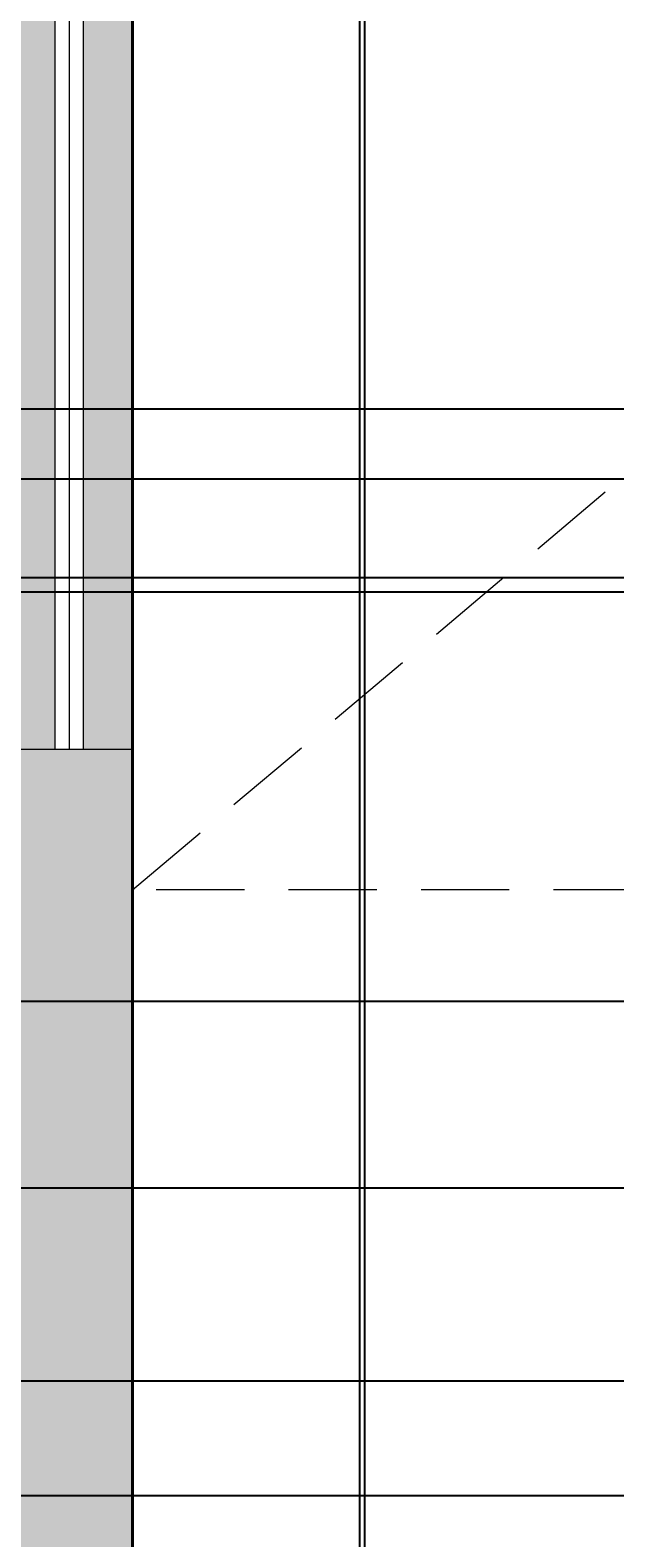
# Model space of a CAD drawing. Units: inches. Extents: x 818 to 1898, y 976 to 2364.
# Tile 67 of 96: x 1260 to 1302, y 1873 to 1980. Entities that reach past the tile are written whole.
import ezdxf

# ---------------------------------------------------------------- set-up
doc = ezdxf.new("R2010")
doc.units = ezdxf.units.IN
doc.header["$LTSCALE"] = 5
doc.header["$MEASUREMENT"] = 0
doc.linetypes.add('HIDDEN', pattern=[0.375, 0.25, -0.125])
for name, color, linetype, lineweight in [('A-ANNO-DIMS', 2, 'Continuous', 18), ('A-FLOR-OVHD', 8, 'HIDDEN', 13), ('A-GLAZ', 4, 'Continuous', 18), ('A-WALL', 7, 'Continuous', 40)]:
    doc.layers.add(name, color=color, linetype=linetype, lineweight=lineweight)
doc.layers.add('A-GLAZ-PATT', color=141, linetype='Continuous', lineweight=9, true_color=0xadddf7)
doc.layers.add('A-WALL-PATT', color=251, linetype='Continuous', lineweight=13, true_color=0x636466)
doc.styles.get("Standard").update_dxf_attribs({"font": 'arial.ttf'})
doc.dimstyles.get("Standard").update_dxf_attribs({"dimtxt": 0.18, "dimasz": 0.18, "dimexe": 0.18, "dimexo": 0.0625, "dimgap": 0.09, "dimtad": 0, "dimtih": 1, "dimtoh": 1, "dimdec": 4, "dimzin": 0, "dimdsep": 46, "dimtxsty": 'Standard', "dimcen": 0.09, "dimadec": 0, "dimazin": 0, "dimtfac": 1, "dimtdec": 4, "dimtofl": 0, "dimtmove": 0, "dimatfit": 3, "dimfxl": 1, "dimtolj": 1, "dimtzin": 0, "dimarcsym": 0})

# ---------------------------------------------------------------- blocks, each defined once
blk = doc.blocks.new('*D61')
at = {"layer": 'A-ANNO-DIMS', "color": 0, "lineweight": -2, "ltscale": 5, "transparency": 16777216}
for p, q in [((1071.73, 1203.03), (1071.73, 2363.87)), ((1071.91, 2363.69), (1250.94, 2363.69)), ((1430.55, 2363.69), (1251.51, 2363.69)), ((1430.73, 1203.03), (1430.73, 2363.87))]:
    blk.add_line(p, q, dxfattribs=at)
at = {"layer": 'A-ANNO-DIMS', "color": 0, "ltscale": 5, "transparency": 16777216}
for points in [[(1071.91, 2363.72), (1071.91, 2363.66), (1071.73, 2363.69)], [(1430.55, 2363.72), (1430.55, 2363.66), (1430.73, 2363.69)]]:
    blk.add_solid(points, dxfattribs=at)
at = {"layer": 'Defpoints', "color": 0, "ltscale": 5, "transparency": 16777216}
for p in [(1430.73, 2363.69), (1071.73, 1202.96), (1430.73, 1202.96)]:
    blk.add_point(p, dxfattribs=at)
at = {"layer": 'A-ANNO-DIMS', "color": 0, "ltscale": 5, "transparency": 16777216, "insert": (1251.23, 2363.69), "char_height": 0.18, "attachment_point": 5}
blk.add_mtext('\\A1;359', dxfattribs=at)
blk = doc.blocks.new('*D64')
at = {"layer": 'A-ANNO-DIMS', "color": 0, "lineweight": -2, "ltscale": 5, "transparency": 16777216}
for p, q in [((1197.73, 1501.14), (1197.73, 2363.87)), ((1197.91, 2363.69), (1313.93, 2363.69)), ((1430.55, 2363.69), (1314.52, 2363.69)), ((1430.73, 1501.14), (1430.73, 2363.87))]:
    blk.add_line(p, q, dxfattribs=at)
at = {"layer": 'A-ANNO-DIMS', "color": 0, "ltscale": 5, "transparency": 16777216}
for points in [[(1197.91, 2363.72), (1197.91, 2363.66), (1197.73, 2363.69)], [(1430.55, 2363.72), (1430.55, 2363.66), (1430.73, 2363.69)]]:
    blk.add_solid(points, dxfattribs=at)
at = {"layer": 'Defpoints', "color": 0, "ltscale": 5, "transparency": 16777216}
for p in [(1430.73, 2363.69), (1197.73, 1501.08), (1430.73, 1501.08)]:
    blk.add_point(p, dxfattribs=at)
at = {"layer": 'A-ANNO-DIMS', "color": 0, "ltscale": 5, "transparency": 16777216, "insert": (1314.23, 2363.69), "char_height": 0.18, "attachment_point": 5}
blk.add_mtext('\\A1;233', dxfattribs=at)
blk = doc.blocks.new('*D74')
at = {"layer": 'A-ANNO-DIMS', "color": 0, "lineweight": -2, "ltscale": 5, "transparency": 16777216}
for p, q in [((1590.66, 1940.08), (818.03, 1940.08)), ((818.21, 1939.9), (818.21, 1925.76)), ((818.21, 1911.26), (818.21, 1925.4)), ((1590.66, 1911.08), (818.03, 1911.08))]:
    blk.add_line(p, q, dxfattribs=at)
at = {"layer": 'A-ANNO-DIMS', "color": 0, "ltscale": 5, "transparency": 16777216}
for points in [[(818.18, 1939.9), (818.24, 1939.9), (818.21, 1940.08)], [(818.18, 1911.26), (818.24, 1911.26), (818.21, 1911.08)]]:
    blk.add_solid(points, dxfattribs=at)
at = {"layer": 'Defpoints', "color": 0, "ltscale": 5, "transparency": 16777216}
for p in [(818.21, 1940.08), (1590.73, 1940.08), (1590.73, 1911.08)]:
    blk.add_point(p, dxfattribs=at)
at = {"layer": 'A-ANNO-DIMS', "color": 0, "ltscale": 5, "transparency": 16777216, "insert": (818.21, 1925.58), "char_height": 0.18, "attachment_point": 5}
blk.add_mtext('\\A1;29', dxfattribs=at)
blk = doc.blocks.new('*D85')
at = {"layer": 'A-ANNO-DIMS', "color": 0, "lineweight": -2, "ltscale": 5, "transparency": 16777216}
for p, q in [((1258.79, 2053.08), (1897.92, 2053.08)), ((1897.74, 2052.9), (1897.74, 1876.76)), ((1897.74, 1700.26), (1897.74, 1876.4)), ((1258.79, 1700.08), (1897.92, 1700.08))]:
    blk.add_line(p, q, dxfattribs=at)
at = {"layer": 'A-ANNO-DIMS', "color": 0, "ltscale": 5, "transparency": 16777216}
for points in [[(1897.71, 2052.9), (1897.77, 2052.9), (1897.74, 2053.08)], [(1897.71, 1700.26), (1897.77, 1700.26), (1897.74, 1700.08)]]:
    blk.add_solid(points, dxfattribs=at)
at = {"layer": 'Defpoints', "color": 0, "ltscale": 5, "transparency": 16777216}
for p in [(1258.73, 2053.08), (1897.74, 2053.08), (1258.73, 1700.08)]:
    blk.add_point(p, dxfattribs=at)
at = {"layer": 'A-ANNO-DIMS', "color": 0, "ltscale": 5, "transparency": 16777216, "insert": (1897.74, 1876.58), "char_height": 0.18, "attachment_point": 5}
blk.add_mtext('\\A1;353', dxfattribs=at)
blk = doc.blocks.new('*D96')
at = {"layer": 'A-ANNO-DIMS', "color": 0, "lineweight": -2, "ltscale": 5, "transparency": 16777216}
for p, q in [((1229.65, 1071.12), (1229.65, 2363.87)), ((1229.83, 2363.69), (1256.52, 2363.69)), ((1283.99, 2363.69), (1257.3, 2363.69)), ((1284.17, 1071.12), (1284.17, 2363.87))]:
    blk.add_line(p, q, dxfattribs=at)
at = {"layer": 'A-ANNO-DIMS', "color": 0, "ltscale": 5, "transparency": 16777216}
for points in [[(1229.83, 2363.72), (1229.83, 2363.66), (1229.65, 2363.69)], [(1283.99, 2363.72), (1283.99, 2363.66), (1284.17, 2363.69)]]:
    blk.add_solid(points, dxfattribs=at)
at = {"layer": 'Defpoints', "color": 0, "ltscale": 5, "transparency": 16777216}
for p in [(1284.17, 2363.69), (1229.65, 1071.06), (1284.17, 1071.06)]:
    blk.add_point(p, dxfattribs=at)
at = {"layer": 'A-ANNO-DIMS', "color": 0, "ltscale": 5, "transparency": 16777216, "insert": (1256.91, 2363.69), "char_height": 0.18, "attachment_point": 5}
blk.add_mtext('\\A1;54.52', dxfattribs=at)
blk = doc.blocks.new('*D97')
at = {"layer": 'A-ANNO-DIMS', "color": 0, "lineweight": -2, "ltscale": 5, "transparency": 16777216}
for p, q in [((1284.17, 1071.12), (1284.17, 2363.87)), ((1284.35, 2363.69), (1310.96, 2363.69)), ((1338.36, 2363.69), (1311.75, 2363.69)), ((1338.54, 1071.12), (1338.54, 2363.87))]:
    blk.add_line(p, q, dxfattribs=at)
at = {"layer": 'A-ANNO-DIMS', "color": 0, "ltscale": 5, "transparency": 16777216}
for points in [[(1284.35, 2363.72), (1284.35, 2363.66), (1284.17, 2363.69)], [(1338.36, 2363.72), (1338.36, 2363.66), (1338.54, 2363.69)]]:
    blk.add_solid(points, dxfattribs=at)
at = {"layer": 'Defpoints', "color": 0, "ltscale": 5, "transparency": 16777216}
for p in [(1338.54, 2363.69), (1284.17, 1071.06), (1338.54, 1071.06)]:
    blk.add_point(p, dxfattribs=at)
at = {"layer": 'A-ANNO-DIMS', "color": 0, "ltscale": 5, "transparency": 16777216, "insert": (1311.36, 2363.69), "char_height": 0.18, "attachment_point": 5}
blk.add_mtext('\\A1;54.37', dxfattribs=at)
blk = doc.blocks.new('*D121')
at = {"layer": 'A-ANNO-DIMS', "color": 0, "lineweight": -2, "ltscale": 5, "transparency": 16777216}
for p, q in [((1766.29, 1884.2), (818.03, 1884.2)), ((818.21, 1884.02), (818.21, 1841.14)), ((818.21, 1797.9), (818.21, 1840.78)), ((1766.29, 1797.72), (818.03, 1797.72))]:
    blk.add_line(p, q, dxfattribs=at)
at = {"layer": 'A-ANNO-DIMS', "color": 0, "ltscale": 5, "transparency": 16777216}
for points in [[(818.18, 1884.02), (818.24, 1884.02), (818.21, 1884.2)], [(818.18, 1797.9), (818.24, 1797.9), (818.21, 1797.72)]]:
    blk.add_solid(points, dxfattribs=at)
at = {"layer": 'Defpoints', "color": 0, "ltscale": 5, "transparency": 16777216}
for p in [(818.21, 1884.2), (1766.35, 1884.2), (1766.35, 1797.72)]:
    blk.add_point(p, dxfattribs=at)
at = {"layer": 'A-ANNO-DIMS', "color": 0, "ltscale": 5, "transparency": 16777216, "insert": (818.21, 1840.96), "char_height": 0.18, "attachment_point": 5}
blk.add_mtext('\\A1;86.49', dxfattribs=at)
blk = doc.blocks.new('*D162')
at = {"layer": 'A-ANNO-DIMS', "color": 0, "lineweight": -2, "ltscale": 5, "transparency": 16777216}
for p, q in [((1429.16, 1876.08), (818.03, 1876.08)), ((818.21, 1875.9), (818.21, 1871.76)), ((818.21, 1867.26), (818.21, 1871.4)), ((1429.16, 1867.08), (818.03, 1867.08))]:
    blk.add_line(p, q, dxfattribs=at)
at = {"layer": 'A-ANNO-DIMS', "color": 0, "ltscale": 5, "transparency": 16777216}
for points in [[(818.18, 1875.9), (818.24, 1875.9), (818.21, 1876.08)], [(818.18, 1867.26), (818.24, 1867.26), (818.21, 1867.08)]]:
    blk.add_solid(points, dxfattribs=at)
at = {"layer": 'Defpoints', "color": 0, "ltscale": 5, "transparency": 16777216}
for p in [(1429.23, 1876.08), (818.21, 1867.08), (1429.23, 1867.08)]:
    blk.add_point(p, dxfattribs=at)
at = {"layer": 'A-ANNO-DIMS', "color": 0, "ltscale": 5, "transparency": 16777216, "insert": (818.21, 1871.58), "char_height": 0.18, "attachment_point": 5}
blk.add_mtext('\\A1;9', dxfattribs=at)
blk = doc.blocks.new('*D165')
at = {"layer": 'A-ANNO-DIMS', "color": 0, "lineweight": -2, "ltscale": 5, "transparency": 16777216}
for p, q in [((1283.82, 1510.14), (1283.82, 2363.87)), ((1284, 2363.69), (1324.09, 2363.69)), ((1364.97, 2363.69), (1324.88, 2363.69)), ((1365.15, 1510.14), (1365.15, 2363.87))]:
    blk.add_line(p, q, dxfattribs=at)
at = {"layer": 'A-ANNO-DIMS', "color": 0, "ltscale": 5, "transparency": 16777216}
for points in [[(1284, 2363.72), (1284, 2363.66), (1283.82, 2363.69)], [(1364.97, 2363.72), (1364.97, 2363.66), (1365.15, 2363.69)]]:
    blk.add_solid(points, dxfattribs=at)
at = {"layer": 'Defpoints', "color": 0, "ltscale": 5, "transparency": 16777216}
for p in [(1365.15, 2363.69), (1283.82, 1510.08), (1365.15, 1510.08)]:
    blk.add_point(p, dxfattribs=at)
at = {"layer": 'A-ANNO-DIMS', "color": 0, "ltscale": 5, "transparency": 16777216, "insert": (1324.48, 2363.69), "char_height": 0.18, "attachment_point": 5}
blk.add_mtext('\\A1;81.33', dxfattribs=at)
blk = doc.blocks.new('*D206')
at = {"layer": 'A-ANNO-DIMS', "color": 0, "lineweight": -2, "ltscale": 5, "transparency": 16777216}
for p, q in [((1590.66, 1911.08), (818.03, 1911.08)), ((818.21, 1910.9), (818.21, 1893.76)), ((818.21, 1876.26), (818.21, 1893.4)), ((1590.66, 1876.08), (818.03, 1876.08))]:
    blk.add_line(p, q, dxfattribs=at)
at = {"layer": 'A-ANNO-DIMS', "color": 0, "ltscale": 5, "transparency": 16777216}
for points in [[(818.18, 1910.9), (818.24, 1910.9), (818.21, 1911.08)], [(818.18, 1876.26), (818.24, 1876.26), (818.21, 1876.08)]]:
    blk.add_solid(points, dxfattribs=at)
at = {"layer": 'Defpoints', "color": 0, "ltscale": 5, "transparency": 16777216}
for p in [(818.21, 1911.08), (1590.73, 1911.08), (1590.73, 1876.08)]:
    blk.add_point(p, dxfattribs=at)
at = {"layer": 'A-ANNO-DIMS', "color": 0, "ltscale": 5, "transparency": 16777216, "insert": (818.21, 1893.58), "char_height": 0.18, "attachment_point": 5}
blk.add_mtext('\\A1;35', dxfattribs=at)
blk = doc.blocks.new('*D211')
at = {"layer": 'A-ANNO-DIMS', "color": 0, "lineweight": -2, "ltscale": 5, "transparency": 16777216}
for p, q in [((1599.66265, 1948.078237), (818.025912, 1948.078237)), ((818.205912, 1947.898237), (818.205912, 1944.758237)), ((818.205912, 1941.258237), (818.205912, 1944.398237)), ((1599.66265, 1941.078237), (818.025912, 1941.078237))]:
    blk.add_line(p, q, dxfattribs=at)
at = {"layer": 'A-ANNO-DIMS', "color": 0, "ltscale": 5, "transparency": 16777216}
for points in [[(818.175912, 1947.898237), (818.235912, 1947.898237), (818.205912, 1948.078237)], [(818.175912, 1941.258237), (818.235912, 1941.258237), (818.205912, 1941.078237)]]:
    blk.add_solid(points, dxfattribs=at)
at = {"layer": 'Defpoints', "color": 0, "ltscale": 5, "transparency": 16777216}
for p in [(818.205912, 1948.078237), (1599.72515, 1948.078237), (1599.72515, 1941.078237)]:
    blk.add_point(p, dxfattribs=at)
at = {"layer": 'A-ANNO-DIMS', "color": 0, "ltscale": 5, "transparency": 16777216, "insert": (818.205912, 1944.578237), "char_height": 0.18, "attachment_point": 5}
blk.add_mtext('\\A1;7', dxfattribs=at)
blk = doc.blocks.new('*D215')
at = {"layer": 'A-ANNO-DIMS', "color": 0, "lineweight": -2, "ltscale": 5, "transparency": 16777216}
for p, q in [((1590.66, 1876.08), (818.03, 1876.08)), ((818.21, 1875.9), (818.21, 1781.76)), ((818.21, 1687.26), (818.21, 1781.4)), ((1511.66, 1687.08), (818.03, 1687.08))]:
    blk.add_line(p, q, dxfattribs=at)
at = {"layer": 'A-ANNO-DIMS', "color": 0, "ltscale": 5, "transparency": 16777216}
for points in [[(818.18, 1875.9), (818.24, 1875.9), (818.21, 1876.08)], [(818.18, 1687.26), (818.24, 1687.26), (818.21, 1687.08)]]:
    blk.add_solid(points, dxfattribs=at)
at = {"layer": 'Defpoints', "color": 0, "ltscale": 5, "transparency": 16777216}
for p in [(818.21, 1876.08), (1590.73, 1876.08), (1511.73, 1687.08)]:
    blk.add_point(p, dxfattribs=at)
at = {"layer": 'A-ANNO-DIMS', "color": 0, "ltscale": 5, "transparency": 16777216, "insert": (818.21, 1781.58), "char_height": 0.18, "attachment_point": 5}
blk.add_mtext('\\A1;189', dxfattribs=at)
blk = doc.blocks.new('*D232')
at = {"layer": 'A-ANNO-DIMS', "color": 0, "lineweight": -2, "ltscale": 5, "transparency": 16777216}
for p, q in [((1303.87, 2008.39), (818.03, 2008.39)), ((818.21, 2008.21), (818.21, 1980.9)), ((818.21, 1953.22), (818.21, 1980.53)), ((1303.87, 1953.04), (818.03, 1953.04))]:
    blk.add_line(p, q, dxfattribs=at)
at = {"layer": 'A-ANNO-DIMS', "color": 0, "ltscale": 5, "transparency": 16777216}
for points in [[(818.18, 2008.21), (818.24, 2008.21), (818.21, 2008.39)], [(818.18, 1953.22), (818.24, 1953.22), (818.21, 1953.04)]]:
    blk.add_solid(points, dxfattribs=at)
at = {"layer": 'Defpoints', "color": 0, "ltscale": 5, "transparency": 16777216}
for p in [(818.21, 2008.39), (1303.93, 2008.39), (1303.93, 1953.04)]:
    blk.add_point(p, dxfattribs=at)
at = {"layer": 'A-ANNO-DIMS', "color": 0, "ltscale": 5, "transparency": 16777216, "insert": (818.21, 1980.72), "char_height": 0.18, "attachment_point": 5}
blk.add_mtext('\\A1;55.35', dxfattribs=at)
blk = doc.blocks.new('*D233')
at = {"layer": 'A-ANNO-DIMS', "color": 0, "lineweight": -2, "ltscale": 5, "transparency": 16777216}
for p, q in [((1267.73, 2044.02), (1267.73, 975.66)), ((1303.93, 2008.33), (1303.93, 975.66)), ((1267.91, 975.84), (1285.36, 975.84)), ((1303.75, 975.84), (1286.29, 975.84))]:
    blk.add_line(p, q, dxfattribs=at)
at = {"layer": 'A-ANNO-DIMS', "color": 0, "ltscale": 5, "transparency": 16777216}
for points in [[(1267.91, 975.87), (1267.91, 975.81), (1267.73, 975.84)], [(1303.75, 975.87), (1303.75, 975.81), (1303.93, 975.84)]]:
    blk.add_solid(points, dxfattribs=at)
at = {"layer": 'Defpoints', "color": 0, "ltscale": 5, "transparency": 16777216}
for p in [(1267.73, 2044.08), (1303.93, 2008.39), (1303.93, 975.84)]:
    blk.add_point(p, dxfattribs=at)
at = {"layer": 'A-ANNO-DIMS', "color": 0, "ltscale": 5, "transparency": 16777216, "insert": (1285.83, 975.84), "char_height": 0.18, "attachment_point": 5}
blk.add_mtext('\\A1;36.206', dxfattribs=at)
blk = doc.blocks.new('*D254')
at = {"layer": 'A-ANNO-DIMS', "color": 0, "lineweight": -2, "ltscale": 5, "transparency": 16777216}
for p, q in [((1267.73, 2044.02), (1267.73, 975.66)), ((1330.3, 2044.02), (1330.3, 975.66)), ((1267.91, 975.84), (1298.62, 975.84)), ((1330.12, 975.84), (1299.41, 975.84))]:
    blk.add_line(p, q, dxfattribs=at)
at = {"layer": 'A-ANNO-DIMS', "color": 0, "ltscale": 5, "transparency": 16777216}
for points in [[(1267.91, 975.87), (1267.91, 975.81), (1267.73, 975.84)], [(1330.12, 975.87), (1330.12, 975.81), (1330.3, 975.84)]]:
    blk.add_solid(points, dxfattribs=at)
at = {"layer": 'Defpoints', "color": 0, "ltscale": 5, "transparency": 16777216}
for p in [(1267.73, 2044.08), (1330.3, 2044.08), (1330.3, 975.84)]:
    blk.add_point(p, dxfattribs=at)
at = {"layer": 'A-ANNO-DIMS', "color": 0, "ltscale": 5, "transparency": 16777216, "insert": (1299.02, 975.84), "char_height": 0.18, "attachment_point": 5}
blk.add_mtext('\\A1;62.58', dxfattribs=at)
blk = doc.blocks.new('*D269')
at = {"layer": 'A-ANNO-DIMS', "color": 0, "lineweight": -2, "ltscale": 5, "transparency": 16777216}
for p, q in [((1246.94, 1534.14), (1246.94, 2363.87)), ((1247.12, 2363.69), (1293.71, 2363.69)), ((1341.08, 2363.69), (1294.49, 2363.69)), ((1341.26, 1534.14), (1341.26, 2363.87))]:
    blk.add_line(p, q, dxfattribs=at)
at = {"layer": 'A-ANNO-DIMS', "color": 0, "ltscale": 5, "transparency": 16777216}
for points in [[(1247.12, 2363.72), (1247.12, 2363.66), (1246.94, 2363.69)], [(1341.08, 2363.72), (1341.08, 2363.66), (1341.26, 2363.69)]]:
    blk.add_solid(points, dxfattribs=at)
at = {"layer": 'Defpoints', "color": 0, "ltscale": 5, "transparency": 16777216}
for p in [(1341.26, 2363.69), (1246.94, 1534.08), (1341.26, 1534.08)]:
    blk.add_point(p, dxfattribs=at)
at = {"layer": 'A-ANNO-DIMS', "color": 0, "ltscale": 5, "transparency": 16777216, "insert": (1294.1, 2363.69), "char_height": 0.18, "attachment_point": 5}
blk.add_mtext('\\A1;94.32', dxfattribs=at)
blk = doc.blocks.new('*D281')
at = {"layer": 'A-ANNO-DIMS', "color": 0, "lineweight": -2, "ltscale": 5, "transparency": 16777216}
for p, q in [((1250.3, 1913.7), (1250.3, 2363.87)), ((1250.48, 2363.69), (1420.12, 2363.69)), ((1590.55, 2363.69), (1420.91, 2363.69)), ((1590.73, 2011.14), (1590.73, 2363.87))]:
    blk.add_line(p, q, dxfattribs=at)
at = {"layer": 'A-ANNO-DIMS', "color": 0, "ltscale": 5, "transparency": 16777216}
for points in [[(1250.48, 2363.72), (1250.48, 2363.66), (1250.3, 2363.69)], [(1590.55, 2363.72), (1590.55, 2363.66), (1590.73, 2363.69)]]:
    blk.add_solid(points, dxfattribs=at)
at = {"layer": 'Defpoints', "color": 0, "ltscale": 5, "transparency": 16777216}
for p in [(1590.73, 2363.69), (1590.73, 2011.08), (1250.3, 1913.64)]:
    blk.add_point(p, dxfattribs=at)
at = {"layer": 'A-ANNO-DIMS', "color": 0, "ltscale": 5, "transparency": 16777216, "insert": (1420.51, 2363.69), "char_height": 0.18, "attachment_point": 5}
blk.add_mtext('\\A1;340.4', dxfattribs=at)
blk = doc.blocks.new('*D287')
at = {"layer": 'A-ANNO-DIMS', "color": 0, "lineweight": -2, "ltscale": 5, "transparency": 16777216}
for p, q in [((1303.87, 1953.04), (818.03, 1953.04)), ((818.21, 1952.86), (818.21, 1925.64)), ((818.21, 1898.05), (818.21, 1925.27)), ((1310.96, 1897.87), (818.03, 1897.87))]:
    blk.add_line(p, q, dxfattribs=at)
at = {"layer": 'A-ANNO-DIMS', "color": 0, "ltscale": 5, "transparency": 16777216}
for points in [[(818.18, 1952.86), (818.24, 1952.86), (818.21, 1953.04)], [(818.18, 1898.05), (818.24, 1898.05), (818.21, 1897.87)]]:
    blk.add_solid(points, dxfattribs=at)
at = {"layer": 'Defpoints', "color": 0, "ltscale": 5, "transparency": 16777216}
for p in [(818.21, 1953.04), (1303.93, 1953.04), (1311.03, 1897.87)]:
    blk.add_point(p, dxfattribs=at)
at = {"layer": 'A-ANNO-DIMS', "color": 0, "ltscale": 5, "transparency": 16777216, "insert": (818.21, 1925.45), "char_height": 0.18, "attachment_point": 5}
blk.add_mtext('\\A1;55.17', dxfattribs=at)

msp = doc.modelspace()

# ---------------------------------------------------------------- hatches: boundary and pattern name
at = {"layer": 'A-GLAZ-PATT', "ltscale": 5}
h = msp.add_hatch(color=256, dxfattribs=at)
h.dxf.hatch_style = 1
h.paths.add_polyline_path([(1283.8183, 1504.5782), (1206.7252, 1504.5782), (1206.7252, 1501.0782), (1283.8183, 1501.0782)])
h.paths.add_polyline_path([(1283.8183, 1510.0782), (1206.7252, 1510.0782), (1206.7252, 1506.5782), (1283.8183, 1506.5782)])
h.paths.add_polyline_path([(1490.9163, 1355.0782), (1439.7252, 1355.0782), (1439.7252, 1409.0522), (1436.2252, 1409.0522), (1436.2252, 1351.5782), (1490.9163, 1351.5782)])
h.paths.add_polyline_path([(1434.2252, 1409.0522), (1430.7251, 1409.0522), (1430.7251, 1346.0782), (1435.0799, 1346.0782), (1435.0731, 1346.1152), (1435.1501, 1346.0782), (1490.9163, 1346.0782), (1490.9163, 1349.5782), (1434.2252, 1349.5782)])
h.paths.add_polyline_path([(1714.7252, 1545.0782), (1711.2252, 1545.0782), (1711.2252, 1521.0782), (1714.7252, 1521.0782)])
h.paths.add_polyline_path([(1709.2252, 1545.0782), (1705.7252, 1545.0782), (1705.7252, 1521.0782), (1709.2252, 1521.0782)])
h.paths.add_polyline_path([(1714.7252, 1687.0782), (1711.2252, 1687.0782), (1711.2252, 1649.9029), (1714.7252, 1649.9029)])
h.paths.add_polyline_path([(1709.2252, 1687.0782), (1705.7252, 1687.0782), (1705.7252, 1649.9029), (1709.2252, 1649.9029)])
h.paths.add_polyline_path([(1709.2252, 1745.5584), (1705.7252, 1745.5584), (1705.7252, 1717.3178), (1709.2252, 1717.3178)])
h.paths.add_polyline_path([(1714.7252, 1745.5584), (1711.2252, 1745.5584), (1711.2252, 1717.3178), (1714.7252, 1717.3178)])
h.paths.add_polyline_path([(1714.7252, 2014.5114), (1711.2252, 2014.5114), (1711.2252, 1962.0338), (1714.7252, 1962.0338)])
h.paths.add_polyline_path([(1709.2252, 2014.5114), (1705.7252, 2014.5114), (1705.7252, 1962.0338), (1709.2252, 1962.0338)])
h.paths.add_polyline_path([(1538.5155, 2047.5782), (1485.1216, 2047.5782), (1485.1216, 2044.0782), (1538.5155, 2044.0782)])
h.paths.add_polyline_path([(1538.5155, 2053.0782), (1485.1216, 2053.0782), (1485.1216, 2049.5782), (1538.5155, 2049.5782)])
h.paths.add_polyline_path([(1388.0315, 2047.5782), (1330.305, 2047.5782), (1330.305, 2044.0782), (1388.0315, 2044.0782)])
h.paths.add_polyline_path([(1388.0315, 2053.0782), (1330.305, 2053.0782), (1330.305, 2049.5782), (1388.0315, 2049.5782)])
h.paths.add_polyline_path([(1262.2252, 2019.2871), (1258.7251, 2019.2871), (1258.7251, 1928.9218), (1262.2252, 1928.9218)])
h.paths.add_polyline_path([(1267.7251, 2019.2871), (1264.2252, 2019.2871), (1264.2252, 1928.9218), (1267.7251, 1928.9218)])
h.paths.add_polyline_path([(1262.2252, 1862.9652), (1258.7251, 1862.9652), (1258.7251, 1814.9652), (1262.2252, 1814.9652)])
h.paths.add_polyline_path([(1267.7251, 1862.9652), (1264.2252, 1862.9652), (1264.2252, 1814.9652), (1267.7251, 1814.9652)])
h.paths.add_polyline_path([(1262.2252, 1755.3321), (1258.7251, 1755.3321), (1258.7251, 1707.3321), (1262.2252, 1707.3321)])
h.paths.add_polyline_path([(1267.7251, 1755.3321), (1264.2252, 1755.3321), (1264.2252, 1707.3321), (1267.7251, 1707.3321)])
h.paths.add_polyline_path([(1251.9333, 1692.5782), (1206.7252, 1692.5782), (1206.7252, 1687.0782), (1251.9333, 1687.0782)])
h.paths.add_polyline_path([(1251.9333, 1700.0782), (1206.7252, 1700.0782), (1206.7252, 1694.5782), (1251.9333, 1694.5782)])
at = {"layer": 'A-WALL-PATT', "ltscale": 5}
h = msp.add_hatch(color=256, dxfattribs=at)
h.dxf.hatch_style = 1
h.paths.add_polyline_path([(1267.7251, 1928.9218), (1258.7251, 1928.9218), (1258.7251, 1913.6401), (1250.3029, 1913.6401), (1250.3029, 1878.3919), (1258.7251, 1878.3919), (1258.7251, 1862.9652), (1267.7251, 1862.9652)])
h.paths.add_polyline_path([(1267.7251, 1814.9652), (1258.7251, 1814.9652), (1258.7251, 1755.3321), (1267.7251, 1755.3321)])
h.paths.add_polyline_path([(1463.7252, 1696.0782), (1267.7251, 1696.0782), (1267.7251, 1707.3321), (1258.7251, 1707.3321), (1258.7251, 1700.0782), (1251.9333, 1700.0782), (1251.9333, 1687.0782), (1463.7252, 1687.0782)])
h.paths.add_polyline_path([(1714.7252, 1717.3178), (1705.7252, 1717.3178), (1705.7252, 1696.0782), (1599.7251, 1696.0782), (1599.7251, 1790.0782), (1705.7252, 1790.0782), (1705.7252, 1785.6125), (1714.7252, 1785.6125), (1714.7252, 1827.2125), (1705.7252, 1827.2125), (1705.7252, 1802.0782), (1599.7251, 1802.0782), (1599.7251, 1867.0782), (1705.7252, 1867.0782), (1705.7252, 1857.2125), (1714.7252, 1857.2125), (1714.7252, 1930.0316), (1741.8409, 1930.0316), (1741.8409, 1935.0316), (1714.7252, 1935.0316), (1714.7252, 1957.0338), (1741.8409, 1957.0338), (1741.8409, 1962.0338), (1714.7252, 1962.0338), (1705.7252, 1962.0338), (1705.7252, 1948.0782), (1599.7251, 1948.0782), (1599.7251, 1981.0782), (1590.7251, 1981.0782), (1590.7251, 1941.0782), (1620.7252, 1941.0782), (1705.7252, 1941.0782), (1705.7252, 1876.0782), (1599.7251, 1876.0782), (1599.7251, 1911.0782), (1590.7251, 1911.0782), (1590.7251, 1876.0782), (1429.2251, 1876.0782), (1429.2251, 1867.0782), (1511.7251, 1867.0782), (1528.593, 1867.0782), (1595.7252, 1867.0782), (1595.7252, 1773.0782), (1520.7252, 1773.0782), (1520.7252, 1837.5823), (1532.593, 1837.5823), (1532.593, 1867.0782), (1528.593, 1867.0782), (1528.593, 1841.5823), (1511.7251, 1841.5823), (1511.7251, 1744.9714), (1520.7252, 1744.9714), (1520.7252, 1761.0782), (1595.7252, 1761.0782), (1595.7252, 1696.0782), (1520.7252, 1696.0782), (1520.7252, 1716.0454), (1511.7251, 1716.0454), (1511.7251, 1696.0782), (1511.7251, 1687.0782), (1714.7252, 1687.0782)])
h.paths.add_polyline_path([(1714.7252, 2053.0782), (1714.7252, 2081.1881), (1709.7252, 2081.1881), (1709.7252, 2053.0782), (1681.6446, 2053.0782), (1681.6446, 2081.1881), (1676.6446, 2081.1881), (1676.6446, 2053.0782), (1538.5155, 2053.0782), (1538.5155, 2044.0782), (1590.7251, 2044.0782), (1590.7251, 2011.0782), (1599.7251, 2011.0782), (1599.7251, 2044.0782), (1705.7252, 2044.0782), (1705.7252, 2014.5114), (1714.7252, 2014.5114)])
h.paths.add_polyline_path([(1485.1216, 2053.0782), (1422.02, 2053.0782), (1422.02, 2081.1881), (1413.02, 2081.1881), (1413.02, 2053.0782), (1399.6356, 2053.0782), (1399.6356, 2081.1881), (1390.6356, 2081.1881), (1390.6356, 2053.0782), (1388.0315, 2053.0782), (1388.0315, 2044.0782), (1416.2743, 2044.0782), (1485.1216, 2044.0782)])
h.paths.add_polyline_path([(1330.305, 2053.0782), (1258.7251, 2053.0782), (1258.7251, 2019.2871), (1267.7251, 2019.2871), (1267.7251, 2044.0782), (1330.305, 2044.0782)])
h.paths.add_polyline_path([(1258.7251, 2053.0782), (1214.6577, 2053.0782), (1214.6577, 2044.0782), (1258.7251, 2044.0782)])
h.paths.add_polyline_path([(1214.6577, 2053.0782), (1180.349, 2053.0782), (1180.349, 2044.0782), (1214.6577, 2044.0782)])
h.paths.add_polyline_path([(1714.7252, 1639.5782), (1741.8409, 1639.5782), (1741.8409, 1643.5782), (1714.7252, 1643.5782), (1714.7252, 1649.9029), (1705.7252, 1649.9029), (1705.7252, 1600.0782), (1477.7252, 1600.0782), (1477.7252, 1591.0782), (1520.7252, 1591.0782), (1616.7252, 1591.0782), (1616.7252, 1416.6857), (1622.7252, 1416.6857), (1622.7252, 1463.0782), (1624.7252, 1463.0782), (1624.7252, 1467.0782), (1622.7252, 1467.0782), (1622.7252, 1591.0782), (1705.7252, 1591.0782), (1705.7252, 1545.0782), (1714.7252, 1545.0782), (1741.8409, 1545.0782), (1741.8409, 1549.0782), (1714.7252, 1549.0782), (1714.7252, 1593.9175), (1737.8409, 1593.9175), (1737.8409, 1597.9175), (1714.7252, 1597.9175)])
h.paths.add_polyline_path([(1674.9024, 2060.7419), (1714.7045, 2060.7419), (1714.7045, 2073.1061), (1674.9024, 2073.1061)], flags=25)
h.paths.add_polyline_path([(1394.5468, 2061.6618), (1422.2344, 2061.6618), (1422.2344, 2074.0261), (1394.5468, 2074.0261)], flags=24)

# ---------------------------------------------------------------- linework, layer by layer
at = {"layer": 'A-FLOR-OVHD', "ltscale": 5}
msp.add_line((1267.7251, 1918.9894), (1416.2743, 2044.0782), dxfattribs=at)
msp.add_lwpolyline([(1267.7251, 2044.0782), (1416.2743, 2044.0782), (1416.2743, 1918.9894), (1267.7251, 1918.9894)], close=True, dxfattribs=at)
at = {"layer": 'A-GLAZ'}
for p, q in [((1262.2252, 2019.2871), (1262.2252, 1928.9218)), ((1263.2252, 2019.2871), (1263.2252, 1928.9218)), ((1264.2252, 2019.2871), (1264.2252, 1928.9218)), ((1267.7251, 1928.9218), (1258.7251, 1928.9218))]:
    msp.add_line(p, q, dxfattribs=at)
at = {"layer": 'A-WALL'}
msp.add_line((1267.7251, 2044.0782), (1267.7251, 1862.9652), dxfattribs=at)

# ---------------------------------------------------------------- dimensions: what is measured, and where the dimension line sits
at = {"layer": 'A-ANNO-DIMS', "ltscale": 5}
for base, p1, p2, override, picture, middle in [((1430.7251, 2363.6929), (1071.7251, 1202.9642), (1430.7251, 1202.9642), {"dimdec": 0, "dimlfac": 1, "dimrnd": 0, "dimzin": 0, "dimdsep": 46, "dimlunit": 2}, '*D61', (1251.2251, 2363.6929)), ((1430.7251, 2363.6929), (1197.7251, 1501.0782), (1430.7251, 1501.0782), {"dimdec": 0, "dimlfac": 1, "dimrnd": 0, "dimzin": 0, "dimdsep": 46, "dimlunit": 2}, '*D64', (1314.2251, 2363.6929)), ((1284.1697, 2363.6929), (1229.6474, 1071.0552), (1284.1697, 1071.0552), {"dimdec": 2, "dimlfac": 1, "dimrnd": 0, "dimzin": 0, "dimdsep": 46, "dimlunit": 2}, '*D96', (1256.9085, 2363.6929)), ((1341.2593, 2363.6929), (1246.9377, 1534.0782), (1341.2593, 1534.0782), {"dimdec": 2, "dimlfac": 1, "dimrnd": 0, "dimzin": 0, "dimdsep": 46, "dimlunit": 2}, '*D269', (1294.0985, 2363.6929)), ((1590.7251, 2363.6929), (1250.3029, 1913.6401), (1590.7251, 2011.0782), {"dimdec": 1, "dimlfac": 1, "dimrnd": 0, "dimzin": 0, "dimdsep": 46, "dimlunit": 2}, '*D281', (1420.514, 2363.6929)), ((1365.1463, 2363.6929), (1283.8183, 1510.0782), (1365.1463, 1510.0782), {"dimdec": 2, "dimlfac": 1, "dimrnd": 0, "dimzin": 0, "dimdsep": 46, "dimlunit": 2}, '*D165', (1324.4823, 2363.6929)), ((1338.5412, 2363.6929), (1284.1697, 1071.0552), (1338.5412, 1071.0552), {"dimdec": 2, "dimlfac": 1, "dimrnd": 0, "dimzin": 0, "dimdsep": 46, "dimlunit": 2}, '*D97', (1311.3554, 2363.6929)), ((1303.9314, 975.8433), (1267.7251, 2044.0782), (1303.9314, 2008.3917), {"dimdec": 3, "dimlfac": 1, "dimrnd": 0, "dimzin": 0, "dimdsep": 46, "dimlunit": 2}, '*D233', (1285.8283, 975.8433)), ((1330.305, 975.8433), (1267.7251, 2044.0782), (1330.305, 2044.0782), {"dimdec": 2, "dimlfac": 1, "dimrnd": 0, "dimzin": 0, "dimdsep": 46, "dimlunit": 2}, '*D254', (1299.0151, 975.8433))]:
    dim = msp.add_linear_dim(base=base, p1=p1, p2=p2, dimstyle='Standard', override=override, dxfattribs=at)
    dim.commit()
    dim.dimension.update_dxf_attribs({"geometry": picture, "text_midpoint": middle})
for base, p1, p2, override, picture, middle in [((1897.736, 2053.0782), (1258.7251, 1700.0782), (1258.7251, 2053.0782), {"dimdec": 0, "dimlfac": 1, "dimrnd": 0, "dimzin": 0, "dimdsep": 46, "dimlunit": 2}, '*D85', (1897.736, 1876.5782)), ((818.2059, 2008.3917), (1303.9314, 1953.0408), (1303.9314, 2008.3917), {"dimdec": 2, "dimlfac": 1, "dimrnd": 0, "dimzin": 0, "dimdsep": 46, "dimlunit": 2}, '*D232', (818.2059, 1980.7163)), ((818.2059, 1953.0408), (1311.025, 1897.8663), (1303.9314, 1953.0408), {"dimdec": 2, "dimlfac": 1, "dimrnd": 0, "dimzin": 0, "dimdsep": 46, "dimlunit": 2}, '*D287', (818.2059, 1925.4536)), ((818.2059, 1948.0782), (1599.7251, 1941.0782), (1599.7251, 1948.0782), {"dimdec": 0, "dimlfac": 1, "dimrnd": 0, "dimzin": 0, "dimdsep": 46, "dimlunit": 2}, '*D211', (818.2059, 1944.5782)), ((818.2059, 1940.0782), (1590.7251, 1911.0782), (1590.7251, 1940.0782), {"dimdec": 0, "dimlfac": 1, "dimrnd": 0, "dimzin": 0, "dimdsep": 46, "dimlunit": 2}, '*D74', (818.2059, 1925.5782)), ((818.2059, 1911.0782), (1590.7251, 1876.0782), (1590.7251, 1911.0782), {"dimdec": 0, "dimlfac": 1, "dimrnd": 0, "dimzin": 0, "dimdsep": 46, "dimlunit": 2}, '*D206', (818.2059, 1893.5782)), ((818.2059, 1884.2031), (1766.3524, 1797.7165), (1766.3524, 1884.2031), {"dimdec": 2, "dimlfac": 1, "dimrnd": 0, "dimzin": 0, "dimdsep": 46, "dimlunit": 2}, '*D121', (818.2059, 1840.9598)), ((818.2059, 1876.0782), (1511.7251, 1687.0782), (1590.7251, 1876.0782), {"dimdec": 0, "dimlfac": 1, "dimrnd": 0, "dimzin": 0, "dimdsep": 46, "dimlunit": 2}, '*D215', (818.2059, 1781.5782)), ((818.2059, 1867.0782), (1429.2251, 1876.0782), (1429.2251, 1867.0782), {"dimdec": 0, "dimlfac": 1, "dimrnd": 0, "dimzin": 0, "dimdsep": 46, "dimlunit": 2}, '*D162', (818.2059, 1871.5782))]:
    dim = msp.add_linear_dim(base=base, p1=p1, p2=p2, angle=90, dimstyle='Standard', override=override, dxfattribs=at)
    dim.commit()
    dim.dimension.update_dxf_attribs({"geometry": picture, "text_midpoint": middle})

doc.saveas('drawing.dxf')
